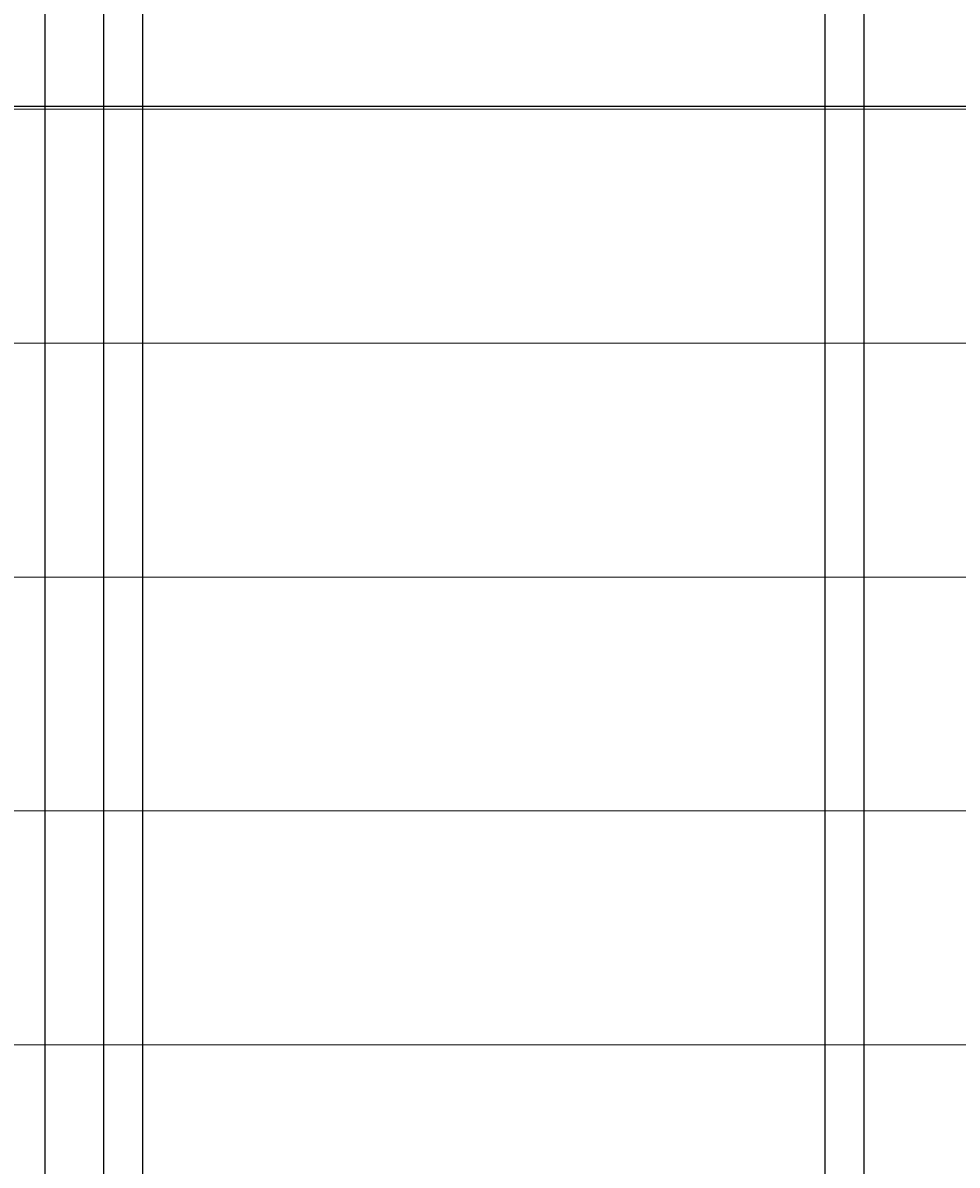
# Model space of a CAD drawing. Units: inches. Extents: x -6 to 289, y -8 to 323.
# Tile 18 of 107: x 126 to 150, y 21 to 50. Entities that reach past the tile are written whole.
import ezdxf

# ---------------------------------------------------------------- set-up
doc = ezdxf.new("R2010")
doc.units = ezdxf.units.IN
doc.header["$MEASUREMENT"] = 0
for name, color, linetype, lineweight in [('A-ANNO-DIMS', 2, 'Continuous', 18), ('A-DOOR', 3, 'Continuous', 25), ('A-ELEV-PATT', 8, 'Continuous', 13)]:
    doc.layers.add(name, color=color, linetype=linetype, lineweight=lineweight)
doc.styles.get("Standard").update_dxf_attribs({"font": 'arial.ttf'})
doc.dimstyles.get("Standard").update_dxf_attribs({"dimtxt": 0.18, "dimasz": 0.18, "dimexe": 0.18, "dimexo": 0.0625, "dimgap": 0.09, "dimtad": 0, "dimtih": 1, "dimtoh": 1, "dimdec": 4, "dimzin": 0, "dimdsep": 46, "dimtxsty": 'Standard', "dimcen": 0.09, "dimadec": 0, "dimazin": 0, "dimtfac": 1, "dimtdec": 4, "dimtofl": 0, "dimtmove": 0, "dimatfit": 3, "dimfxl": 1, "dimtolj": 1, "dimtzin": 0, "dimarcsym": 0})

# ---------------------------------------------------------------- blocks, each defined once
blk = doc.blocks.new('*D16')
at = {"layer": 'A-ANNO-DIMS', "color": 0, "lineweight": -2, "transparency": 16777216}
for p, q in [((9.943, 68.37), (9.943, -8.391)), ((272.973, 68.37), (272.973, -8.391)), ((10.123, -8.211), (140.993, -8.211)), ((272.793, -8.211), (141.923, -8.211))]:
    blk.add_line(p, q, dxfattribs=at)
at = {"layer": 'A-ANNO-DIMS', "color": 0, "transparency": 16777216}
for points in [[(10.123, -8.181), (10.123, -8.241), (9.943, -8.211)], [(272.793, -8.181), (272.793, -8.241), (272.973, -8.211)]]:
    blk.add_solid(points, dxfattribs=at)
at = {"layer": 'Defpoints', "color": 0, "transparency": 16777216}
for p in [(9.943, 68.432), (272.973, 68.432), (272.973, -8.211)]:
    blk.add_point(p, dxfattribs=at)
at = {"layer": 'A-ANNO-DIMS', "color": 0, "transparency": 16777216, "insert": (141.458, -8.211), "char_height": 0.18, "attachment_point": 5}
blk.add_mtext('\\A1;263.03', dxfattribs=at)
blk = doc.blocks.new('*D28')
at = {"layer": 'A-ANNO-DIMS', "color": 0, "lineweight": -2, "transparency": 16777216}
for p, q in [((128.383, 180.092), (128.383, -8.391)), ((126.883, 178.592), (126.883, -8.391)), ((127.063, -8.211), (127.387, -8.211)), ((128.203, -8.211), (127.88, -8.211))]:
    blk.add_line(p, q, dxfattribs=at)
at = {"layer": 'A-ANNO-DIMS', "color": 0, "transparency": 16777216}
for points in [[(127.063, -8.181), (127.063, -8.241), (126.883, -8.211)], [(128.203, -8.181), (128.203, -8.241), (128.383, -8.211)]]:
    blk.add_solid(points, dxfattribs=at)
at = {"layer": 'Defpoints', "color": 0, "transparency": 16777216}
for p in [(128.383, 180.154), (126.883, 178.654), (128.383, -8.211)]:
    blk.add_point(p, dxfattribs=at)
at = {"layer": 'A-ANNO-DIMS', "color": 0, "transparency": 16777216, "insert": (127.633, -8.211), "char_height": 0.18, "attachment_point": 5}
blk.add_mtext('\\A1;1.5', dxfattribs=at)
blk = doc.blocks.new('*D29')
at = {"layer": 'A-ANNO-DIMS', "color": 0, "lineweight": -2, "transparency": 16777216}
for p, q in [((129.383, 181.092), (129.383, -8.391)), ((128.383, 180.092), (128.383, -8.391)), ((128.563, -8.211), (128.76, -8.211)), ((129.203, -8.211), (129.007, -8.211))]:
    blk.add_line(p, q, dxfattribs=at)
at = {"layer": 'A-ANNO-DIMS', "color": 0, "transparency": 16777216}
for points in [[(128.563, -8.181), (128.563, -8.241), (128.383, -8.211)], [(129.203, -8.181), (129.203, -8.241), (129.383, -8.211)]]:
    blk.add_solid(points, dxfattribs=at)
at = {"layer": 'Defpoints', "color": 0, "transparency": 16777216}
for p in [(129.383, 181.154), (128.383, 180.154), (129.383, -8.211)]:
    blk.add_point(p, dxfattribs=at)
at = {"layer": 'A-ANNO-DIMS', "color": 0, "transparency": 16777216, "insert": (128.883, -8.211), "char_height": 0.18, "attachment_point": 5}
blk.add_mtext('\\A1;1', dxfattribs=at)
blk = doc.blocks.new('*D30')
at = {"layer": 'A-ANNO-DIMS', "color": 0, "lineweight": -2, "transparency": 16777216}
for p, q in [((129.383, 181.092), (129.383, -8.391)), ((146.883, 181.092), (146.883, -8.391)), ((129.563, -8.211), (137.817, -8.211)), ((146.703, -8.211), (138.449, -8.211))]:
    blk.add_line(p, q, dxfattribs=at)
at = {"layer": 'A-ANNO-DIMS', "color": 0, "transparency": 16777216}
for points in [[(129.563, -8.181), (129.563, -8.241), (129.383, -8.211)], [(146.703, -8.181), (146.703, -8.241), (146.883, -8.211)]]:
    blk.add_solid(points, dxfattribs=at)
at = {"layer": 'Defpoints', "color": 0, "transparency": 16777216}
for p in [(129.383, 181.154), (146.883, 181.154), (146.883, -8.211)]:
    blk.add_point(p, dxfattribs=at)
at = {"layer": 'A-ANNO-DIMS', "color": 0, "transparency": 16777216, "insert": (138.133, -8.211), "char_height": 0.18, "attachment_point": 5}
blk.add_mtext('\\A1;17.5', dxfattribs=at)
blk = doc.blocks.new('*D31')
at = {"layer": 'A-ANNO-DIMS', "color": 0, "lineweight": -2, "transparency": 16777216}
for p, q in [((146.883, 181.092), (146.883, -8.391)), ((147.883, 181.092), (147.883, -8.391)), ((147.063, -8.211), (147.26, -8.211)), ((147.703, -8.211), (147.507, -8.211))]:
    blk.add_line(p, q, dxfattribs=at)
at = {"layer": 'A-ANNO-DIMS', "color": 0, "transparency": 16777216}
for points in [[(147.063, -8.181), (147.063, -8.241), (146.883, -8.211)], [(147.703, -8.181), (147.703, -8.241), (147.883, -8.211)]]:
    blk.add_solid(points, dxfattribs=at)
at = {"layer": 'Defpoints', "color": 0, "transparency": 16777216}
for p in [(146.883, 181.154), (147.883, 181.154), (147.883, -8.211)]:
    blk.add_point(p, dxfattribs=at)
at = {"layer": 'A-ANNO-DIMS', "color": 0, "transparency": 16777216, "insert": (147.383, -8.211), "char_height": 0.18, "attachment_point": 5}
blk.add_mtext('\\A1;1', dxfattribs=at)
blk = doc.blocks.new('*D32')
at = {"layer": 'A-ANNO-DIMS', "color": 0, "lineweight": -2, "transparency": 16777216}
for p, q in [((147.883, 181.092), (147.883, -8.391)), ((166.383, 181.092), (166.383, -8.391)), ((148.063, -8.211), (156.817, -8.211)), ((166.203, -8.211), (157.449, -8.211))]:
    blk.add_line(p, q, dxfattribs=at)
at = {"layer": 'A-ANNO-DIMS', "color": 0, "transparency": 16777216}
for points in [[(148.063, -8.181), (148.063, -8.241), (147.883, -8.211)], [(166.203, -8.181), (166.203, -8.241), (166.383, -8.211)]]:
    blk.add_solid(points, dxfattribs=at)
at = {"layer": 'Defpoints', "color": 0, "transparency": 16777216}
for p in [(147.883, 181.154), (166.383, 181.154), (166.383, -8.211)]:
    blk.add_point(p, dxfattribs=at)
at = {"layer": 'A-ANNO-DIMS', "color": 0, "transparency": 16777216, "insert": (157.133, -8.211), "char_height": 0.18, "attachment_point": 5}
blk.add_mtext('\\A1;18.5', dxfattribs=at)

msp = doc.modelspace()

# ---------------------------------------------------------------- hatches: boundary and pattern name
at = {"layer": 'A-ELEV-PATT'}
h = msp.add_hatch(dxfattribs=at)
h.set_pattern_fill('_USER', color=256, scale=6, pattern_type=0)
h.set_pattern_definition([(0, (0, 0), (0, 6), [])])
h.paths.add_polyline_path([(184.1244, 48.0851), (124.008, 48.0851), (124.008, 10.2888), (184.1244, 10.2888)])
h.paths.add_polyline_path([(244.2408, 48.0851), (186.3604, 48.0851), (186.3604, 10.2888), (244.2408, 10.2888)])
h.paths.add_polyline_path([(208.2918, 114.2795), (190.7918, 114.2795), (190.7918, 71.2795), (208.2918, 71.2795)])
h.paths.add_polyline_path([(227.7918, 114.2795), (209.2918, 114.2795), (209.2918, 71.2795), (227.7918, 71.2795)])
h.paths.add_polyline_path([(211.2918, 224.3887), (190.7918, 224.3887), (190.7918, 162.3484), (211.2918, 162.3484)])
h.paths.add_polyline_path([(233.7918, 224.3887), (212.2918, 224.3887), (212.2918, 162.3484), (233.7918, 162.3484)])
h.paths.add_polyline_path([(166.3835, 224.154), (147.8835, 224.154), (147.8835, 181.154), (166.3835, 181.154)])
h.paths.add_polyline_path([(146.8835, 224.154), (129.3835, 224.154), (129.3835, 181.154), (146.8835, 181.154)])

# ---------------------------------------------------------------- linework, layer by layer
at = {"layer": 'A-DOOR'}
msp.add_lwpolyline([(124.008, 48.0851), (244.2408, 48.0851), (244.2408, 10.2888), (124.008, 10.2888)], close=True, dxfattribs=at)

# ---------------------------------------------------------------- dimensions: what is measured, and where the dimension line sits
at = {"layer": 'A-ANNO-DIMS'}
for base, p1, p2, override, picture, middle in [((129.3835, -8.2112), (128.3835, 180.154), (129.3835, 181.154), {"dimdec": 0, "dimlfac": 1, "dimrnd": 0, "dimzin": 0, "dimdsep": 46, "dimlunit": 2}, '*D29', (128.8835, -8.2112)), ((146.8835, -8.2112), (129.3835, 181.154), (146.8835, 181.154), {"dimdec": 1, "dimlfac": 1, "dimrnd": 0, "dimzin": 0, "dimdsep": 46, "dimlunit": 2}, '*D30', (138.1335, -8.2112)), ((147.8835, -8.2112), (146.8835, 181.154), (147.8835, 181.154), {"dimdec": 0, "dimlfac": 1, "dimrnd": 0, "dimzin": 0, "dimdsep": 46, "dimlunit": 2}, '*D31', (147.3835, -8.2112)), ((166.3835, -8.2112), (147.8835, 181.154), (166.3835, 181.154), {"dimdec": 1, "dimlfac": 1, "dimrnd": 0, "dimzin": 0, "dimdsep": 46, "dimlunit": 2}, '*D32', (157.1335, -8.2112)), ((128.3835, -8.2112), (126.8835, 178.654), (128.3835, 180.154), {"dimdec": 1, "dimlfac": 1, "dimrnd": 0, "dimzin": 0, "dimdsep": 46, "dimlunit": 2}, '*D28', (127.6335, -8.2112)), ((272.9733, -8.2112), (9.943, 68.4322), (272.9733, 68.4322), {"dimdec": 2, "dimlfac": 1, "dimrnd": 0, "dimzin": 0, "dimdsep": 46, "dimlunit": 2}, '*D16', (141.4581, -8.2112))]:
    dim = msp.add_linear_dim(base=base, p1=p1, p2=p2, dimstyle='Standard', override=override, dxfattribs=at)
    dim.commit()
    dim.dimension.update_dxf_attribs({"geometry": picture, "text_midpoint": middle})

doc.saveas('drawing.dxf')
